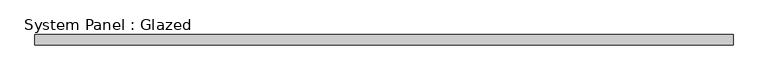
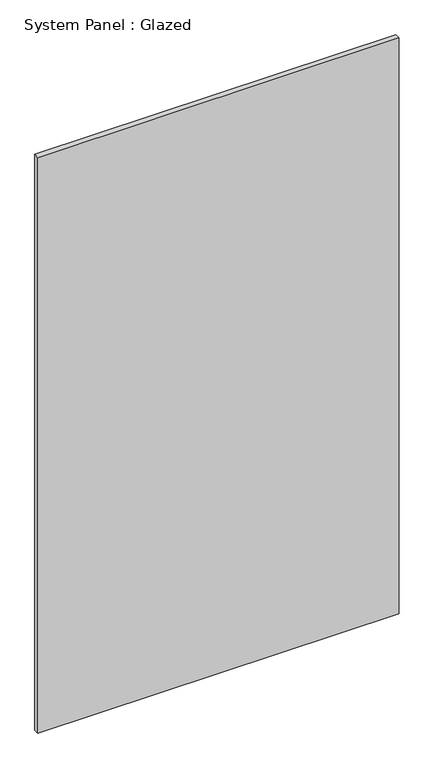
"""IFC4 building model written with IfcOpenShell, lengths in millimetres: plate geometry, System Panel : Glazed."""

from ifc_helpers import new_model, si_unit, origin, origin_with_axes, place, context, project, spatial, polyline, outline, extrude, source, transform, mapped, element, save


def system_panel_glazed_5e65faa0(model_context):
    return source(origin(), model_context, "Body", "SweptSolid", [
        extrude(outline(polyline([(866.775, 19.05), (-866.775, 19.05), (-866.775, 44.45), (866.775, 44.45), (866.775, 19.05)])), origin_with_axes(), (0.0, 0.0, 1.0), 2921.0),
    ])


if __name__ == "__main__":
    model = new_model("IFC4")
    model_context = context("Model", 3, world=origin())
    ifc_project = project(units=[si_unit("LENGTHUNIT", "METRE", prefix="MILLI")], contexts=[model_context])
    site = spatial("IfcSite", under=ifc_project)
    building = spatial("IfcBuilding", under=site)
    placement = place(None, origin())
    system_panel_glazed_shape = system_panel_glazed_5e65faa0(model_context)
    element("IfcPlate", 1, ObjectType="System Panel : Glazed", at=placement, inside=building, context=model_context, shape_type="MappedRepresentation", body=[
        mapped(system_panel_glazed_shape, transform((0.0, 0.0, 0.0), x_axis=(1.0, 0.0, 0.0), y_axis=(0.0, 1.0, 0.0), z_axis=(0.0, 0.0, 1.0))),
    ])
    save(model, "model.ifc")

# Revit data of these elements
# Type "System Panel : Glazed"
#   Construction Type Id = "GSP4R"
#   Analytic Construction = "1/8 in Pilkington single glazing"
#   Visual Light Transmittance = 0.9
#   Solar Heat Gain Coefficient = 0.86
#   Heat Transfer Coefficient (U) = 1.18115 BTU/(h·ft²·°F)
# Element 1 (IfcPlate, "System Panel : Glazed")
#   Materials on its faces: "Glass"
# Materials
#   "Glass": class "Glass", colour RGB 0 128 192, transparency 0.75, Description = "Soda Lime Glass", Cost = 0
